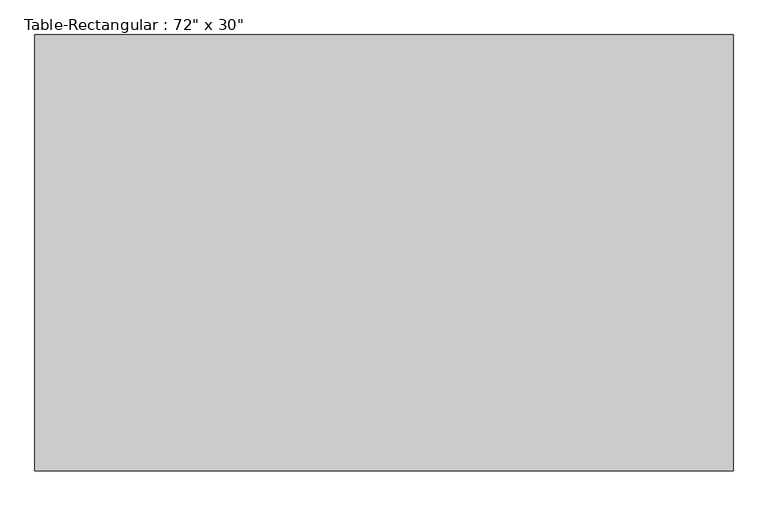
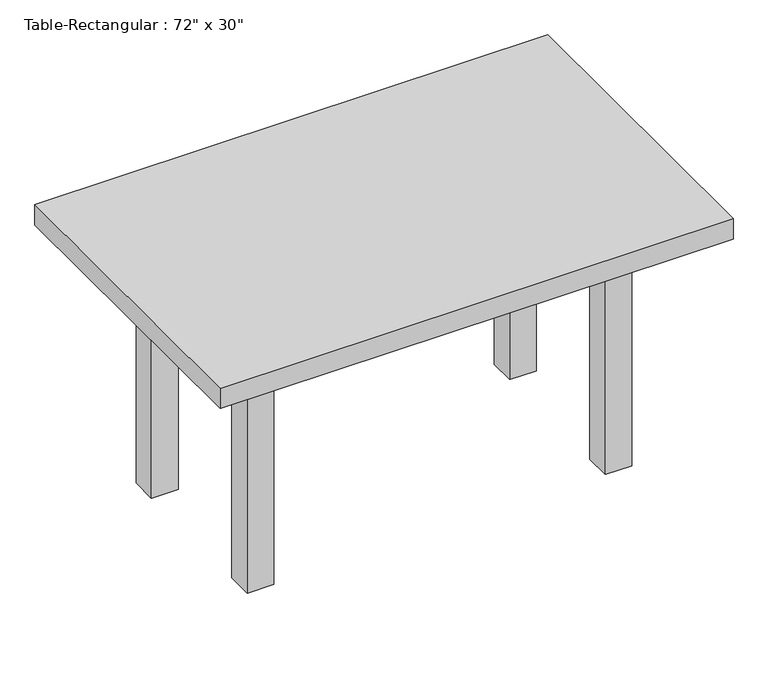
"""IFC4 building model written with IfcOpenShell, lengths in millimetres: furniture geometry."""

from ifc_helpers import new_model, si_unit, frame, origin, origin_with_axes, place, context, project, spatial, polyline, outline, extrude, source, transform, mapped, element, save


def furniture_3f969c1c(model_context):
    return source(origin(), model_context, "Body", "SweptSolid", [
        extrude(outline(polyline([(393.7, 190.5), (393.7, 165.1), (-393.7, 165.1), (-393.7, 190.5), (393.7, 190.5)])), frame((0.0, 0.0, 508.0), z_axis=(0.0, 0.0, 1.0), x_axis=(1.0, 0.0, 0.0)), (0.0, 0.0, 1.0), 101.6),
        extrude(outline(polyline([(393.7, -190.5), (-393.7, -190.5), (-393.7, -165.1), (393.7, -165.1), (393.7, -190.5)])), frame((0.0, 0.0, 508.0), z_axis=(0.0, 0.0, 1.0), x_axis=(1.0, 0.0, 0.0)), (0.0, 0.0, 1.0), 101.6),
        extrude(outline(polyline([(-406.4, -165.1), (-431.8, -165.1), (-431.8, 165.1), (-406.4, 165.1), (-406.4, -165.1)])), frame((0.0, 0.0, 508.0), z_axis=(0.0, 0.0, 1.0), x_axis=(1.0, 0.0, 0.0)), (0.0, 0.0, 1.0), 101.6),
        extrude(outline(polyline([(406.4, -165.1), (406.4, 165.1), (431.8, 165.1), (431.8, -165.1), (406.4, -165.1)])), frame((0.0, 0.0, 508.0), z_axis=(0.0, 0.0, 1.0), x_axis=(1.0, 0.0, 0.0)), (0.0, 0.0, 1.0), 101.6),
        extrude(outline(polyline([(609.6, 381.0), (609.6, -381.0), (-609.6, -381.0), (-609.6, 381.0), (609.6, 381.0)])), frame((0.0, 0.0, 609.6), z_axis=(0.0, 0.0, 1.0), x_axis=(1.0, 0.0, 0.0)), (0.0, 0.0, 1.0), 50.8),
        extrude(outline(polyline([(-393.7, 228.6), (-393.7, 165.1), (-457.2, 165.1), (-457.2, 228.6), (-393.7, 228.6)])), origin_with_axes(), (0.0, 0.0, 1.0), 609.6),
        extrude(outline(polyline([(393.7, 228.6), (457.2, 228.6), (457.2, 165.1), (393.7, 165.1), (393.7, 228.6)])), origin_with_axes(), (0.0, 0.0, 1.0), 609.6),
        extrude(outline(polyline([(-393.7, -228.6), (-457.2, -228.6), (-457.2, -165.1), (-393.7, -165.1), (-393.7, -228.6)])), origin_with_axes(), (0.0, 0.0, 1.0), 609.6),
        extrude(outline(polyline([(393.7, -228.6), (393.7, -165.1), (457.2, -165.1), (457.2, -228.6), (393.7, -228.6)])), origin_with_axes(), (0.0, 0.0, 1.0), 609.6),
    ])


if __name__ == "__main__":
    model = new_model("IFC4")
    model_context = context("Model", 3, world=origin())
    ifc_project = project(units=[si_unit("LENGTHUNIT", "METRE", prefix="MILLI")], contexts=[model_context])
    site = spatial("IfcSite", under=ifc_project)
    building = spatial("IfcBuilding", under=site)
    placement = place(None, origin())
    furniture_shape = furniture_3f969c1c(model_context)
    element("IfcFurniture", 1, ObjectType="Table-Rectangular : 72\" x 30\"", at=placement, inside=building, context=model_context, shape_type="MappedRepresentation", body=[
        mapped(furniture_shape, transform((0.0, 0.0, 0.0), x_axis=(1.0, 0.0, 0.0), y_axis=(0.0, 1.0, 0.0), z_axis=(0.0, 0.0, 1.0))),
    ])
    save(model, "model.ifc")

# Revit data of these elements
# Type "Table-Rectangular : 72\" x 30\""
#   Assembly Code = "E2020200"
#   Height = 2' - 2"
#   Length = 4' - 0"
#   Width = 2' - 6"
#   Base Material = Birch
#   Top Material = Birch
#   Default Elevation = 0
# Element 1 (IfcFurniture, "Table-Rectangular : 72\" x 30\"")
#   Materials on its faces: "Birch"
# Materials
#   "Birch": class "Wood", colour RGB 224 178 126, transparency 0, Description = "Betula Alleghaniensis", Cost = 0
